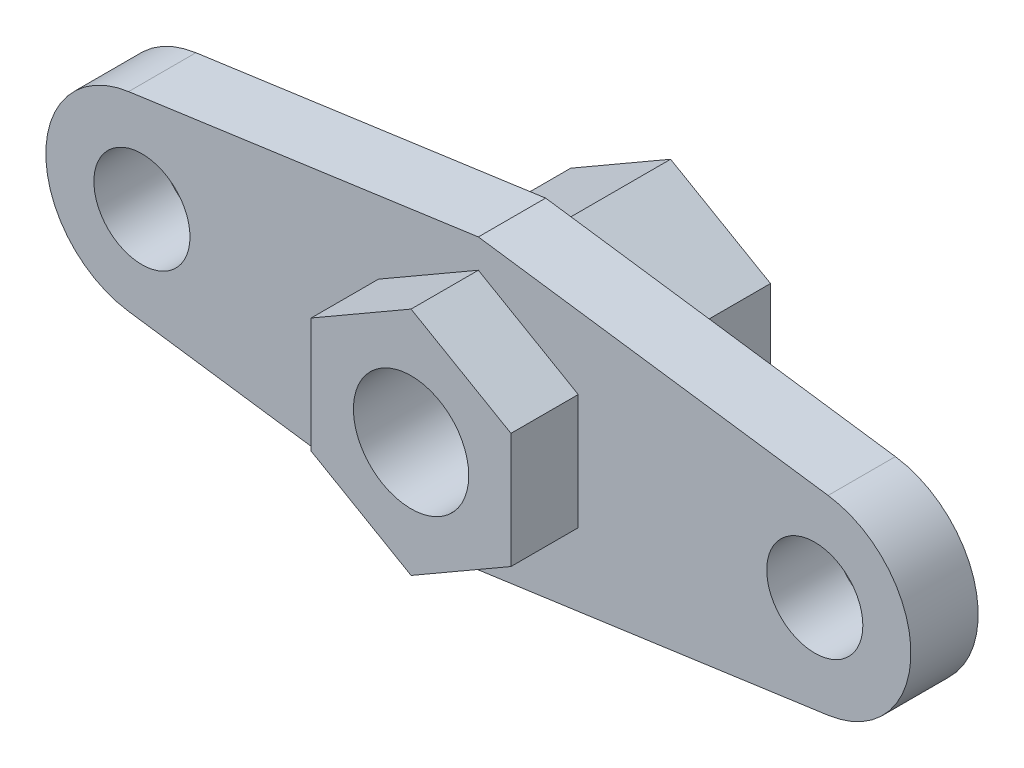
SolidWorks part; units mm, degrees
material "Plain Carbon Steel"
ref_plane "Front Plane" through (0, 0, 0) normal (0, 0, 1) x (1, 0, 0)
ref_plane "Top Plane" through (0, 0, 0) normal (0, 1, 0) x (1, 0, 0)
ref_plane "Right Plane" through (0, 0, 0) normal (1, 0, 0) x (0, 0, -1)
sketch "Link Plate Profile" plane through (0, 0, 0) normal (0, 0, 1) x (1, 0, 0)
  line L0 (-15.4348, 0) -> (54.5652, 0) construction
  line L3 (19.5652, 15) -> (-16.8219, 9.9033)
  line L10 (19.5652, 12) -> (9.1729, 6)
  line L11 (9.1729, 6) -> (9.1729, -6)
  line L12 (9.1729, -6) -> (19.5652, -12)
  line L13 (19.5652, -12) -> (29.9575, -6)
  line L14 (29.9575, -6) -> (29.9575, 6)
  line L15 (29.9575, 6) -> (19.5652, 12)
  line L16 (19.5652, 15) -> (55.9524, 9.9033)
  line L18 (55.9524, -9.9033) -> (19.5652, -15)
  line L19 (-16.8219, -9.9033) -> (19.5652, -15)
  arc A0 (-15.4348, 10) -> (-15.4348, -10) centre (-15.4348, 0) ccw
  arc A1 (54.5652, -10) -> (54.5652, 10) centre (54.5652, 0) ccw
  circle A2 centre (-15.4348, 0) radius 5
  circle A3 centre (19.5652, 0) radius 12 construction
  circle A4 centre (19.5652, 0) radius 6
  circle A5 centre (54.5652, 0) radius 5
  point P3 (19.5652, 0)
  dimension "D1" = 10
  dimension "D3" = 10
  dimension "D5" = 12
  dimension "D6" = 10
  dimension "D7" = 10
  dimension "D2" = 70
  dimension "D4" = 12
  dimension "D8" = 15
  dimension "D9" = 15.4348
extrude "Link Plate" add sketch "Link Plate Profile" along normal mid plane 7
sketch "Front Hex Profile" plane through (0, 0, 0) normal (0, 0, 1) x (1, 0, 0)
  line L0 (9.1729, 6) -> (9.1729, -6) construction
  line L1 (9.1729, -6) -> (19.5652, -12) construction
  line L2 (19.5652, -12) -> (29.9575, -6) construction
  line L3 (29.9575, -6) -> (29.9575, 6) construction
  line L4 (29.9575, 6) -> (19.5652, 12) construction
  line L5 (19.5652, 12) -> (9.1729, 6) construction
  line L6 (9.1729, 6) -> (9.1729, -6)
  line L7 (9.1729, -6) -> (19.5652, -12)
  line L8 (19.5652, -12) -> (29.9575, -6)
  line L9 (29.9575, -6) -> (29.9575, 6)
  line L10 (29.9575, 6) -> (19.5652, 12)
  line L11 (19.5652, 12) -> (9.1729, 6)
extrude "Front Hex Boss" add sketch "Front Hex Profile" along normal blind 10.5
sketch "Rear Hex Profile" plane through (0, 0, 0) normal (0, 0, -1) x (-1, 0, 0)
  line L6 (-9.1729, 6) -> (-19.5652, 12)
  line L7 (-19.5652, 12) -> (-29.9575, 6)
  line L8 (-29.9575, 6) -> (-29.9575, -6)
  line L9 (-29.9575, -6) -> (-19.5652, -12)
  line L10 (-19.5652, -12) -> (-9.1729, -6)
  line L11 (-9.1729, -6) -> (-9.1729, 6)
  line L12 (-9.1729, 6) -> (-19.5652, 12)
  line L13 (-19.5652, 12) -> (-29.9575, 6)
  line L14 (-29.9575, 6) -> (-29.9575, -6)
  line L15 (-29.9575, -6) -> (-19.5652, -12)
  line L16 (-19.5652, -12) -> (-9.1729, -6)
  line L17 (-9.1729, -6) -> (-9.1729, 6)
  dimension "D1" = 0
extrude "Rear Hex Boss" add sketch "Rear Hex Profile" along normal blind 16.5
sketch "Centre Bore Profile" plane through (0, 0, 10.5) normal (0, 0, 1) x (1, 0, 0)
  line L0 (9.1729, 6) -> (9.1729, -6) construction
  circle A0 centre (19.5652, 0) radius 6
  dimension "D1" = 12
  dimension "D2" = 10.3923
  dimension "D3" = 12
extrude "Centre Bore Ø12" cut sketch "Centre Bore Profile" against normal through all
